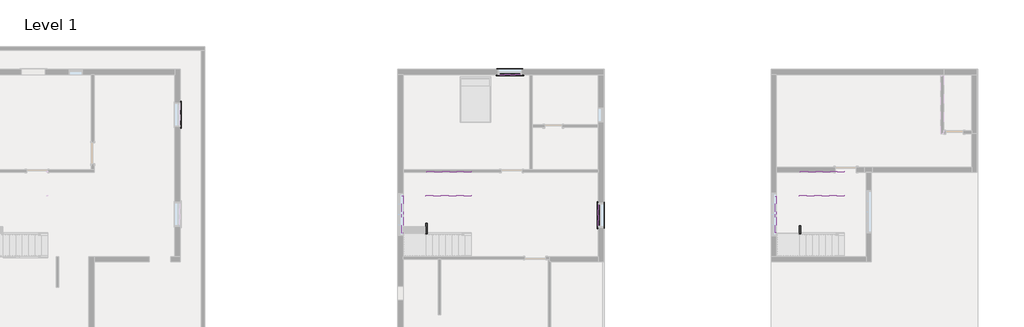
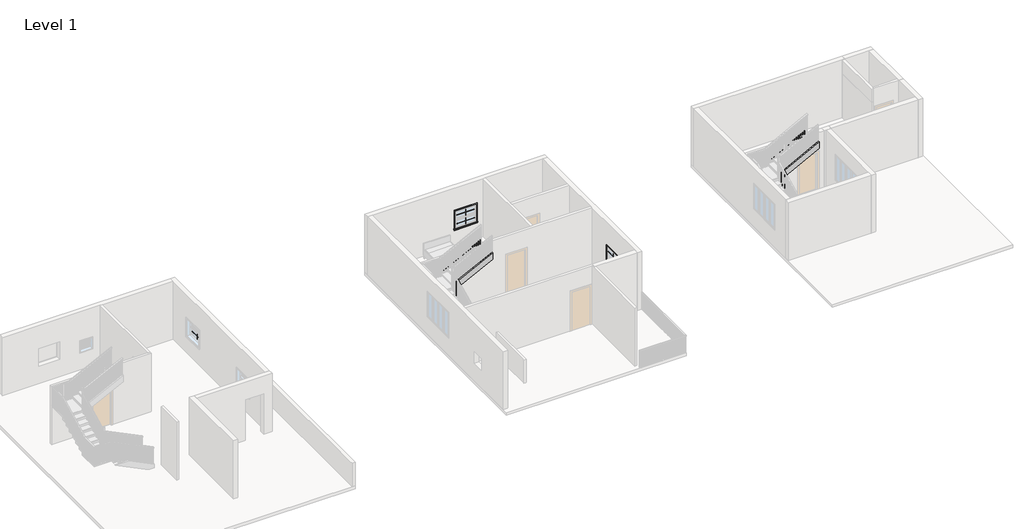
# One storey, part 8 of 8: 10 proxies, 8 members.
"""IFC4 building model written with IfcOpenShell, lengths in millimetres."""

from ifc_helpers import new_model, si_unit, frame, origin, place, context, project, spatial, polyline, outline, extrude, transform, mapped, element, save
from components import muntin_pattern_2x2_muntin_pattern_2x2_4e6d5dbc, muntin_pattern_2x2_muntin_pattern_2x2_9ec9cf3e, trim_window_exterior_flat_with_sill_79aa6636, trim_window_interior_flat_picture_frame_55a9d760

model = new_model("IFC4")

# Units and contexts
model_context = context("Model", 3, world=origin())
ifc_project = project(units=[si_unit("LENGTHUNIT", "METRE", prefix="MILLI")], contexts=[model_context])

# Site, building, storey
site = spatial("IfcSite", under=ifc_project)
building = spatial("IfcBuilding", under=site)
storey = spatial("IfcBuildingStorey", under=building, Name="Level 1", Elevation=0.0)

# Proxies
placement = place(None, origin())
muntin_pattern_2x2_muntin_pattern_2x2_shape = muntin_pattern_2x2_muntin_pattern_2x2_4e6d5dbc(model_context)
element("IfcBuildingElementProxy", 1, Name="Muntin Pattern_2x2 : Muntin Pattern_2x2", ObjectType="Muntin Pattern_2x2 : Muntin Pattern_2x2", at=placement, inside=storey, context=model_context, shape_type="MappedRepresentation", body=[
    mapped(muntin_pattern_2x2_muntin_pattern_2x2_shape, transform((4093.1941518, 681.7850713, 1441.45), x_axis=(0.0, 1.0, 0.0), y_axis=(-1.0, 0.0, 0.0), z_axis=(0.0, 0.0, 1.0))),
])
element("IfcBuildingElementProxy", 2, Name="Muntin Pattern_2x2 : Muntin Pattern_2x2", ObjectType="Muntin Pattern_2x2 : Muntin Pattern_2x2", at=placement, inside=storey, context=model_context, shape_type="MappedRepresentation", body=[
    mapped(muntin_pattern_2x2_muntin_pattern_2x2_shape, transform((254.6191518, 6777.7850713, 1441.45), x_axis=(-1.0, 0.0, 0.0), y_axis=(0.0, -1.0, 0.0), z_axis=(0.0, 0.0, 1.0))),
])
muntin_pattern_2x2_muntin_pattern_2x2_2_shape = muntin_pattern_2x2_muntin_pattern_2x2_9ec9cf3e(model_context)
element("IfcBuildingElementProxy", 3, Name="Muntin Pattern_2x2 : Muntin Pattern_2x2", ObjectType="Muntin Pattern_2x2 : Muntin Pattern_2x2", at=placement, inside=storey, context=model_context, shape_type="MappedRepresentation", body=[
    mapped(muntin_pattern_2x2_muntin_pattern_2x2_2_shape, transform((-14039.0039184, 5028.3600713, 984.25), x_axis=(0.0, -1.0, 0.0), y_axis=(1.0, 0.0, 0.0), z_axis=(0.0, 0.0, 1.0))),
])
element("IfcBuildingElementProxy", 4, Name="Muntin Pattern_2x2 : Muntin Pattern_2x2", ObjectType="Muntin Pattern_2x2 : Muntin Pattern_2x2", at=placement, inside=storey, context=model_context, shape_type="MappedRepresentation", body=[
    mapped(muntin_pattern_2x2_muntin_pattern_2x2_2_shape, transform((4093.1941518, 681.7850713, 984.25), x_axis=(0.0, 1.0, 0.0), y_axis=(-1.0, 0.0, 0.0), z_axis=(0.0, 0.0, 1.0))),
])
element("IfcBuildingElementProxy", 5, Name="Muntin Pattern_2x2 : Muntin Pattern_2x2", ObjectType="Muntin Pattern_2x2 : Muntin Pattern_2x2", at=placement, inside=storey, context=model_context, shape_type="MappedRepresentation", body=[
    mapped(muntin_pattern_2x2_muntin_pattern_2x2_2_shape, transform((254.6191518, 6777.7850713, 984.25), x_axis=(-1.0, 0.0, 0.0), y_axis=(0.0, -1.0, 0.0), z_axis=(0.0, 0.0, 1.0))),
])
trim_window_exterior_flat_with_sill_shape = trim_window_exterior_flat_with_sill_79aa6636(model_context)
element("IfcBuildingElementProxy", 6, Name="Trim-Window-Exterior-Flat : with Sill", ObjectType="Trim-Window-Exterior-Flat : with Sill", at=placement, inside=storey, context=model_context, shape_type="MappedRepresentation", body=[
    mapped(trim_window_exterior_flat_with_sill_shape, transform((-14029.4789184, 5028.3600713, 1828.8), x_axis=(0.0, 1.0, 0.0), y_axis=(0.0, 0.0, 1.0), z_axis=(1.0, 0.0, 0.0))),
])
element("IfcBuildingElementProxy", 7, Name="Trim-Window-Exterior-Flat : with Sill", ObjectType="Trim-Window-Exterior-Flat : with Sill", at=placement, inside=storey, context=model_context, shape_type="MappedRepresentation", body=[
    mapped(trim_window_exterior_flat_with_sill_shape, transform((4083.6691518, 681.7850713, 1828.8), x_axis=(0.0, -1.0, 0.0), y_axis=(0.0, 0.0, 1.0), z_axis=(-1.0, 0.0, 0.0))),
])
element("IfcBuildingElementProxy", 8, Name="Trim-Window-Exterior-Flat : with Sill", ObjectType="Trim-Window-Exterior-Flat : with Sill", at=placement, inside=storey, context=model_context, shape_type="MappedRepresentation", body=[
    mapped(trim_window_exterior_flat_with_sill_shape, transform((254.6191518, 6768.2600713, 1828.8), x_axis=(1.0, 0.0, 0.0), y_axis=(0.0, 0.0, 1.0), z_axis=(0.0, -1.0, 0.0))),
])
trim_window_interior_flat_picture_frame_shape = trim_window_interior_flat_picture_frame_55a9d760(model_context)
element("IfcBuildingElementProxy", 9, Name="Trim-Window-Interior-Flat : Picture Frame", ObjectType="Trim-Window-Interior-Flat : Picture Frame", at=placement, inside=storey, context=model_context, shape_type="MappedRepresentation", body=[
    mapped(trim_window_interior_flat_picture_frame_shape, transform((4312.2691518, 681.7850713, 1828.8), x_axis=(0.0, 1.0, 0.0), y_axis=(0.0, 0.0, 1.0), z_axis=(1.0, 0.0, 0.0))),
])
element("IfcBuildingElementProxy", 10, Name="Trim-Window-Interior-Flat : Picture Frame", ObjectType="Trim-Window-Interior-Flat : Picture Frame", at=placement, inside=storey, context=model_context, shape_type="MappedRepresentation", body=[
    mapped(trim_window_interior_flat_picture_frame_shape, transform((254.6191518, 6996.8600713, 1828.8), x_axis=(-1.0, 0.0, 0.0), y_axis=(0.0, 0.0, 1.0), z_axis=(0.0, 1.0, 0.0))),
])

# Members
element("IfcMember", 11, ObjectType="Stringer - 2\" Width", at=placement, inside=storey, context=model_context, shape_type="SweptSolid", body=[
    extrude(outline(polyline([(-102.7408997, 1323.6027923), (837.3600713, 1789.768563), (1523.4610422, 1789.768563), (583.3600713, 1323.6027923), (-102.7408997, 1323.6027923)])), frame((-4425.3308482, 0.0, 0.0), z_axis=(1.0, 0.0, 0.0), x_axis=(0.0, 1.0, 0.0)), (0.0, 0.0, 1.0), 50.8),
])
element("IfcMember", 12, ObjectType="Stringer - 2\" Width", at=placement, inside=storey, context=model_context, shape_type="SweptSolid", body=[
    extrude(outline(polyline([(2293.4209741, -2672.7308482), (2910.5779989, -1428.1308482), (3250.7933564, -1428.1308482), (2293.4209741, -3358.8318192), (2293.4209741, -2672.7308482)])), frame((0.0, 2539.1600713, 0.0), z_axis=(0.0, 1.0, 0.0), x_axis=(0.0, 0.0, 1.0)), (0.0, 0.0, 1.0), 50.8),
])
element("IfcMember", 13, ObjectType="Stringer - 2\" Width", at=placement, inside=storey, context=model_context, shape_type="SweptSolid", body=[
    extrude(outline(polyline([(-127.8399287, 970.9416352), (-127.8399287, 1311.1569927), (1497.7600713, 2117.2396374), (1497.7600713, 1777.0242799), (-127.8399287, 970.9416352)])), frame((-3383.9308482, 0.0, 0.0), z_axis=(1.0, 0.0, 0.0), x_axis=(0.0, 1.0, 0.0)), (0.0, 0.0, 1.0), 50.8),
])
element("IfcMember", 14, ObjectType="Stringer - 2\" Width", at=placement, inside=storey, context=model_context, shape_type="SweptSolid", body=[
    extrude(outline(polyline([(2280.9751746, -3383.9308482), (1940.759817, -3383.9308482), (2910.5779989, -1428.1308482), (3250.7933564, -1428.1308482), (2280.9751746, -3383.9308482)])), frame((0.0, 1497.7600713, 0.0), z_axis=(0.0, 1.0, 0.0), x_axis=(0.0, 0.0, 1.0)), (0.0, 0.0, 1.0), 50.8),
])
element("IfcMember", 15, ObjectType="Stringer - 2\" Width", at=placement, inside=storey, context=model_context, shape_type="SweptSolid", body=[
    extrude(outline(polyline([(-77.8258841, 1391.7469745), (837.3600713, 1867.1682501), (1498.5460266, 1867.1682501), (583.3600713, 1391.7469745), (-77.8258841, 1391.7469745)])), frame((11753.042447, 0.0, 0.0), z_axis=(1.0, 0.0, 0.0), x_axis=(0.0, 1.0, 0.0)), (0.0, 0.0, 1.0), 50.8),
])
element("IfcMember", 16, ObjectType="Stringer - 2\" Width", at=placement, inside=storey, context=model_context, shape_type="SweptSolid", body=[
    extrude(outline(polyline([(2407.7469745, 13505.642447), (3054.2924291, 14750.242447), (3397.7656526, 14750.242447), (2407.7469745, 12844.4564917), (2407.7469745, 13505.642447)])), frame((0.0, 2539.1600713, 0.0), z_axis=(0.0, 1.0, 0.0), x_axis=(0.0, 0.0, 1.0)), (0.0, 0.0, 1.0), 50.8),
])
element("IfcMember", 17, ObjectType="Stringer - 2\" Width", at=placement, inside=storey, context=model_context, shape_type="SweptSolid", body=[
    extrude(outline(polyline([(-127.8399287, 1022.2924291), (-127.8399287, 1365.7656526), (1497.7600713, 2210.2331851), (1497.7600713, 1866.7599615), (-127.8399287, 1022.2924291)])), frame((12794.442447, 0.0, 0.0), z_axis=(1.0, 0.0, 0.0), x_axis=(0.0, 1.0, 0.0)), (0.0, 0.0, 1.0), 50.8),
])
element("IfcMember", 18, ObjectType="Stringer - 2\" Width", at=placement, inside=storey, context=model_context, shape_type="SweptSolid", body=[
    extrude(outline(polyline([(2381.7656526, 12794.442447), (2038.2924291, 12794.442447), (3054.2924291, 14750.242447), (3397.7656526, 14750.242447), (2381.7656526, 12794.442447)])), frame((0.0, 1497.7600713, 0.0), z_axis=(0.0, 1.0, 0.0), x_axis=(0.0, 0.0, 1.0)), (0.0, 0.0, 1.0), 50.8),
])

save(model, "model.ifc")

# Revit data of these elements
# Type "Muntin Pattern_2x2 : Muntin Pattern_2x2"
#   Width [instance default] = 4' - 0"
#   Thickness = 0' - 0 1/2"
#   Height [instance default] = 4' - 0"
#   Distance = 0' - 0 3/4"
#   Interior Material [instance default] = none
#   Exterior Material [instance default] = none
#   Default Elevation = 0
# Type "Trim-Window-Exterior-Flat : with Sill"
#   Trim Width = 0' - 2 1/4"
#   Trim Thickness_Picture Frame = 0' - 1 1/4"
#   Trim Thickness_with Sill = 0' - 0 3/4"
#   Sill Thickness = 0' - 1 1/4"
#   Opening Width [instance default] = 2' - 0"
#   Opening Height [instance default] = 3' - 0"
#   Default Elevation = 4' - 0"
#   Sill = yes
#   Picture Frame = no
#   Trim Material [instance default] = none
# Type "Trim-Window-Interior-Flat : Picture Frame"
#   Trim Thickness_Picture Frame = 0' - 1 1/4"
#   Trim Width = 0' - 2 1/4"
#   Trim Thickness_with Sill = 0' - 0 3/4"
#   Sill Thickness = 0' - 1 1/4"
#   Opening Width [instance default] = 2' - 0"
#   Opening Height [instance default] = 3' - 0"
#   Default Elevation = 4' - 0"
#   Sill = no
#   Picture Frame = yes
#   Trim Material [instance default] = none
# Elements 1, 2 (IfcBuildingElementProxy, "Muntin Pattern_2x2 : Muntin Pattern_2x2")
#   Width = 2' - 11 1/2"
#   Height = 1' - 0 1/2"
#   Interior Material = Wood - Stained
#   Exterior Material = Clad - White
#   Phase Created = New Construction
#   Materials on its faces: "Clad - White", "Wood - Stained"
# Elements 3, 4, 5 (IfcBuildingElementProxy, "Muntin Pattern_2x2 : Muntin Pattern_2x2")
#   Width = 2' - 11 1/2"
#   Height = 1' - 0.49965"
#   Interior Material = Wood - Stained
#   Exterior Material = Clad - White
#   Phase Created = New Construction
#   Materials on its faces: "Clad - White", "Wood - Stained"
# Elements 6, 7, 8 (IfcBuildingElementProxy, "Trim-Window-Exterior-Flat : with Sill")
#   Opening Width = 3' - 5"
#   Opening Height = 3' - 0"
#   Trim Material = Clad - White
#   Phase Created = New Construction
#   Materials on its faces: "Clad - White"
# Elements 9, 10 (IfcBuildingElementProxy, "Trim-Window-Interior-Flat : Picture Frame")
#   Opening Width = 3' - 5"
#   Opening Height = 3' - 0"
#   Trim Material = Wood - Stained
#   Phase Created = New Construction
#   Materials on its faces: "Wood - Stained"
# Elements 11, 12, 13, 14, 15, 16, 17, 18 (IfcMember, "Stringer - 2\" Width")
#   Phase Created = New Construction
# Materials
#   "Clad - White": class "Wood", colour RGB 242 242 238, transparency 0, Cost = 0
#   "Wood - Stained": class "Wood", colour RGB 224 178 126, transparency 0, Cost = 0
